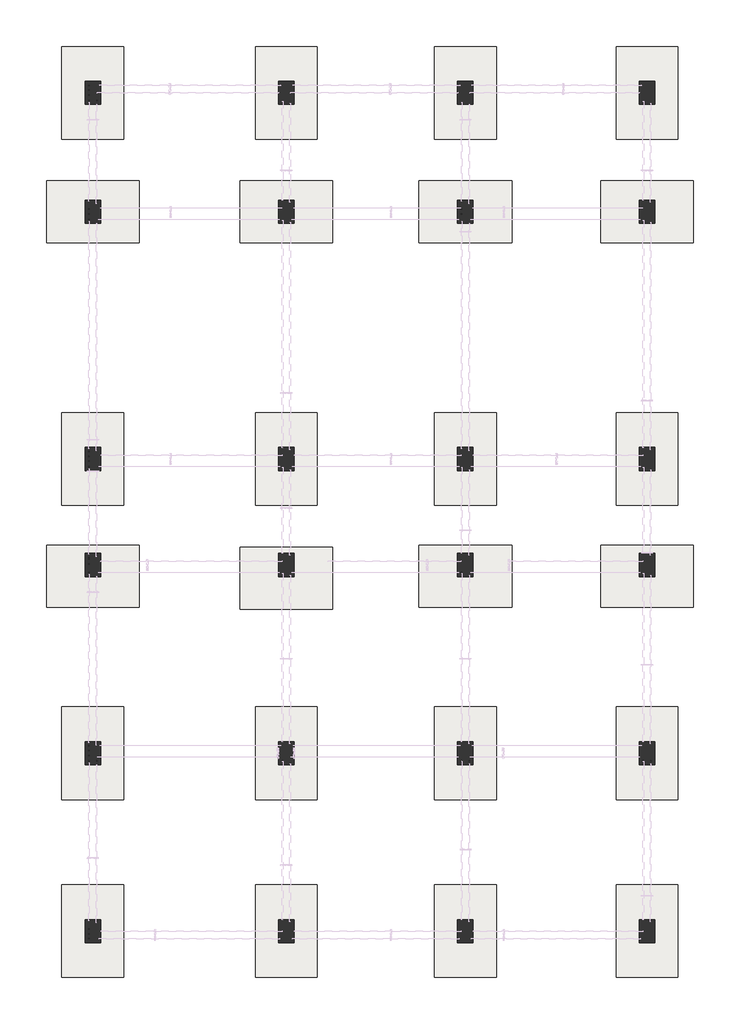
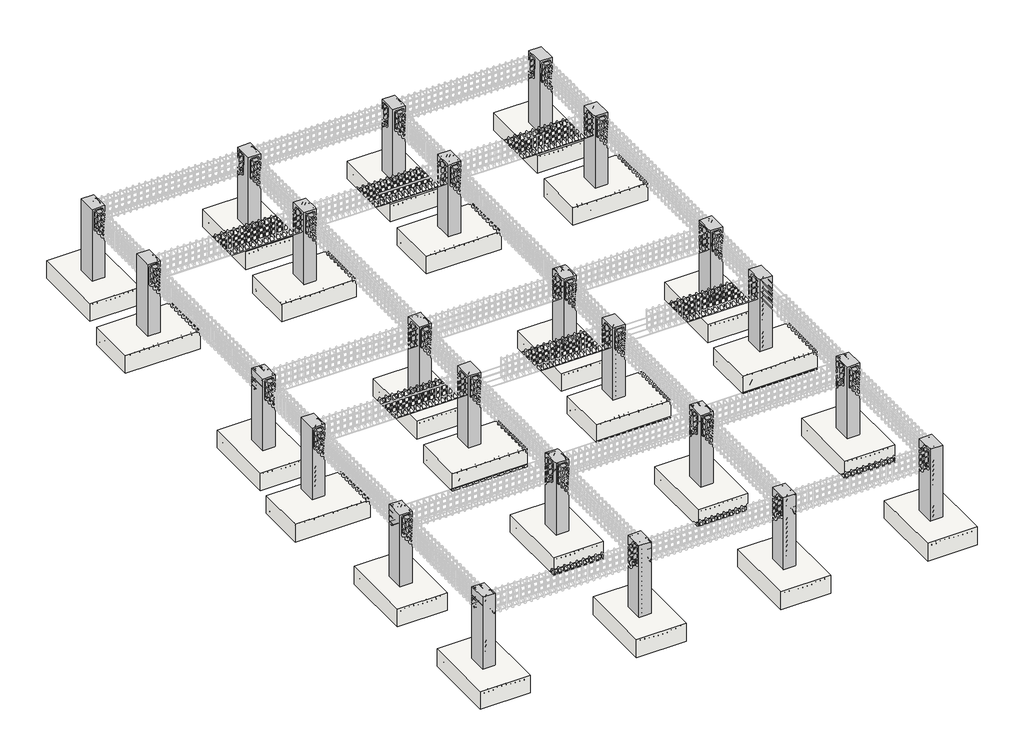
# One storey, part 1 of 20: 24 columns, 24 slabs.
"""IFC4 building model written with IfcOpenShell, lengths in millimetres."""

from ifc_helpers import new_model, si_unit, frame, origin, place, context, project, spatial, polyline, outline, extrude, faceted_brep, transform, mapped, element, save
from components import m_footing_rectangular_1800_x_1200_x_450mm_16ba7ea5

model = new_model("IFC4")

# Units and contexts
model_context = context("Model", 3, world=origin())
ifc_project = project(units=[si_unit("LENGTHUNIT", "METRE", prefix="MILLI")], contexts=[model_context])

# Site, building, storey
site = spatial("IfcSite", under=ifc_project)
building = spatial("IfcBuilding", under=site)
storey = spatial("IfcBuildingStorey", under=building, Elevation=-1828.8)

# Columns
placement = place(None, origin())
element("IfcColumn", 1, ObjectType="M_Concrete-Rectangular-Column : 300 x 450mm", at=placement, inside=storey, context=model_context, shape_type="Brep", body=[
    faceted_brep([(-5713.9412236, 10327.3331363, -1828.8), (-5713.9412236, 9877.3331363, -1828.8), (-6013.9412236, 9877.3331363, -1828.8), (-6013.9412236, 10327.3331363, -1828.8), (-5713.9412236, 10327.3331363, 0.0), (-5713.9412236, 10027.3331363, 0.0), (-5713.9412236, 9877.3331363, 0.0), (-6013.9412236, 9877.3331363, 0.0), (-6013.9412236, 10327.3331363, 0.0)], [[[0, 1, 2, 3]], [[4, 5, 6, 1, 0]], [[6, 7, 2, 1]], [[7, 8, 3, 2]], [[8, 4, 0, 3]], [[4, 8, 7, 6, 5]]]),
])
element("IfcColumn", 2, ObjectType="M_Concrete-Rectangular-Column : 300 x 450mm", at=placement, inside=storey, context=model_context, shape_type="Brep", body=[
    faceted_brep([(-5713.9412236, 8015.9331363, -1828.8), (-5713.9412236, 7565.9331363, -1828.8), (-6013.9412236, 7565.9331363, -1828.8), (-6013.9412236, 8015.9331363, -1828.8), (-5713.9412236, 8015.9331363, 0.0), (-5713.9412236, 7940.9331363, 0.0), (-5713.9412236, 7640.9331363, 0.0), (-5713.9412236, 7565.9331363, 0.0), (-6013.9412236, 7565.9331363, 0.0), (-6013.9412236, 8015.9331363, 0.0)], [[[0, 1, 2, 3]], [[4, 5, 6, 7, 1, 0]], [[7, 8, 2, 1]], [[8, 9, 3, 2]], [[9, 4, 0, 3]], [[4, 9, 8, 7, 6, 5]]]),
])
element("IfcColumn", 3, ObjectType="M_Concrete-Rectangular-Column : 300 x 450mm", at=placement, inside=storey, context=model_context, shape_type="Brep", body=[
    faceted_brep([(-5713.9412236, 3215.3331363, -1828.8), (-5713.9412236, 2765.3331363, -1828.8), (-6013.9412236, 2765.3331363, -1828.8), (-6013.9412236, 3215.3331363, -1828.8), (-5713.9412236, 3215.3331363, 0.0), (-5713.9412236, 3140.3331363, 0.0), (-5713.9412236, 2840.3331363, 0.0), (-5713.9412236, 2765.3331363, 0.0), (-6013.9412236, 2765.3331363, 0.0), (-6013.9412236, 3215.3331363, 0.0)], [[[0, 1, 2, 3]], [[4, 5, 6, 7, 1, 0]], [[7, 8, 2, 1]], [[8, 9, 3, 2]], [[9, 4, 0, 3]], [[4, 9, 8, 7, 6, 5]]]),
])
element("IfcColumn", 4, ObjectType="M_Concrete-Rectangular-Column : 300 x 450mm", at=placement, inside=storey, context=model_context, shape_type="Brep", body=[
    faceted_brep([(-6013.9412236, 707.9331363, -1828.8), (-6013.9412236, 1157.9331363, -1828.8), (-5713.9412236, 1157.9331363, -1828.8), (-5713.9412236, 707.9331363, -1828.8), (-6013.9412236, 707.9331363, 0.0), (-6013.9412236, 1157.9331363, 0.0), (-5713.9412236, 1157.9331363, 0.0), (-5713.9412236, 782.9331363, 0.0), (-5713.9412236, 707.9331363, 0.0)], [[[0, 1, 2, 3]], [[4, 5, 1, 0]], [[5, 6, 2, 1]], [[6, 7, 8, 3, 2]], [[8, 4, 0, 3]], [[4, 8, 7, 6, 5]]]),
])
element("IfcColumn", 5, ObjectType="M_Concrete-Rectangular-Column : 300 x 450mm", at=placement, inside=storey, context=model_context, shape_type="Brep", body=[
    faceted_brep([(-5713.9412236, -2499.6668637, -1828.8), (-5713.9412236, -2949.6668637, -1828.8), (-6013.9412236, -2949.6668637, -1828.8), (-6013.9412236, -2499.6668637, -1828.8), (-5713.9412236, -2499.6668637, 0.0), (-5713.9412236, -2574.6668637, 0.0), (-5713.9412236, -2874.6668637, 0.0), (-5713.9412236, -2949.6668637, 0.0), (-6013.9412236, -2949.6668637, 0.0), (-6013.9412236, -2499.6668637, 0.0)], [[[0, 1, 2, 3]], [[4, 5, 6, 7, 1, 0]], [[7, 8, 2, 1]], [[8, 9, 3, 2]], [[9, 4, 0, 3]], [[4, 9, 8, 7, 6, 5]]]),
])
element("IfcColumn", 6, ObjectType="M_Concrete-Rectangular-Column : 300 x 450mm", at=placement, inside=storey, context=model_context, shape_type="Brep", body=[
    faceted_brep([(-6013.9412236, -6404.0668637, -1828.8), (-6013.9412236, -5954.0668637, -1828.8), (-5713.9412236, -5954.0668637, -1828.8), (-5713.9412236, -6404.0668637, -1828.8), (-6013.9412236, -6404.0668637, 0.0), (-6013.9412236, -5954.0668637, 0.0), (-5713.9412236, -5954.0668637, 0.0), (-5713.9412236, -6104.0668637, 0.0), (-5713.9412236, -6404.0668637, 0.0)], [[[0, 1, 2, 3]], [[4, 5, 1, 0]], [[5, 6, 2, 1]], [[6, 7, 8, 3, 2]], [[8, 4, 0, 3]], [[4, 8, 7, 6, 5]]]),
])
element("IfcColumn", 7, ObjectType="M_Concrete-Rectangular-Column : 300 x 450mm", at=placement, inside=storey, context=model_context, shape_type="Brep", body=[
    faceted_brep([(-1952.7860107, 10327.3331363, -1828.8), (-1952.7860107, 9877.3331363, -1828.8), (-2252.7860107, 9877.3331363, -1828.8), (-2252.7860107, 10327.3331363, -1828.8), (-1952.7860107, 10327.3331363, 0.0), (-1952.7860107, 10027.3331363, 0.0), (-1952.7860107, 9877.3331363, 0.0), (-1952.7860107, 9877.3331363, -300.0), (-2252.7860107, 9877.3331363, 0.0), (-2252.7860107, 9877.3331363, -300.0), (-2252.7860107, 10027.3331363, 0.0), (-2252.7860107, 10327.3331363, 0.0)], [[[0, 1, 2, 3]], [[1, 0, 4, 5, 6, 7]], [[2, 1, 7, 6, 8, 9]], [[3, 2, 9, 8, 10, 11]], [[0, 3, 11, 4]], [[8, 6, 5, 4, 11, 10]]]),
])
element("IfcColumn", 8, ObjectType="M_Concrete-Rectangular-Column : 300 x 450mm", at=placement, inside=storey, context=model_context, shape_type="Brep", body=[
    faceted_brep([(-1952.7860107, 8015.9331363, -1828.8), (-1952.7860107, 7565.9331363, -1828.8), (-2252.7860107, 7565.9331363, -1828.8), (-2252.7860107, 8015.9331363, -1828.8), (-1952.7860107, 8015.9331363, -300.0), (-1952.7860107, 8015.9331363, 0.0), (-1952.7860107, 7940.9331363, 0.0), (-1952.7860107, 7640.9331363, 0.0), (-1952.7860107, 7565.9331363, 0.0), (-1952.7860107, 7565.9331363, -300.0), (-2252.7860107, 7565.9331363, 0.0), (-2252.7860107, 7565.9331363, -300.0), (-2252.7860107, 7640.9331363, 0.0), (-2252.7860107, 7940.9331363, 0.0), (-2252.7860107, 8015.9331363, 0.0), (-2252.7860107, 8015.9331363, -300.0)], [[[0, 1, 2, 3]], [[1, 0, 4, 5, 6, 7, 8, 9]], [[2, 1, 9, 8, 10, 11]], [[3, 2, 11, 10, 12, 13, 14, 15]], [[0, 3, 15, 14, 5, 4]], [[10, 8, 7, 6, 5, 14, 13, 12]]]),
])
element("IfcColumn", 9, ObjectType="M_Concrete-Rectangular-Column : 300 x 450mm", at=placement, inside=storey, context=model_context, shape_type="Brep", body=[
    faceted_brep([(-1952.7860107, 3215.3331363, -1828.8), (-1952.7860107, 2765.3331363, -1828.8), (-2252.7860107, 2765.3331363, -1828.8), (-2252.7860107, 3215.3331363, -1828.8), (-1952.7860107, 3215.3331363, -300.0), (-1952.7860107, 3215.3331363, 0.0), (-1952.7860107, 3140.3331363, 0.0), (-1952.7860107, 2765.3331363, 0.0), (-2252.7860107, 2765.3331363, 0.0), (-2252.7860107, 2765.3331363, -300.0), (-2252.7860107, 2840.3331363, 0.0), (-2252.7860107, 3140.3331363, 0.0), (-2252.7860107, 3215.3331363, 0.0), (-2252.7860107, 3215.3331363, -300.0)], [[[0, 1, 2, 3]], [[1, 0, 4, 5, 6, 7]], [[2, 1, 7, 8, 9]], [[3, 2, 9, 8, 10, 11, 12, 13]], [[0, 3, 13, 12, 5, 4]], [[8, 7, 6, 5, 12, 11, 10]]]),
])
element("IfcColumn", 10, ObjectType="M_Concrete-Rectangular-Column : 300 x 450mm", at=placement, inside=storey, context=model_context, shape_type="Brep", body=[
    faceted_brep([(-2252.7860107, 707.9331363, -1828.8), (-2252.7860107, 1157.9331363, -1828.8), (-1952.7860107, 1157.9331363, -1828.8), (-1952.7860107, 707.9331363, -1828.8), (-2252.7860107, 707.9331363, -300.0), (-2252.7860107, 707.9331363, 0.0), (-2252.7860107, 782.9331363, 0.0), (-2252.7860107, 1082.9331363, 0.0), (-2252.7860107, 1157.9331363, 0.0), (-2252.7860107, 1157.9331363, -300.0), (-1952.7860107, 1157.9331363, 0.0), (-1952.7860107, 782.9331363, 0.0), (-1952.7860107, 707.9331363, 0.0), (-1952.7860107, 707.9331363, -300.0)], [[[0, 1, 2, 3]], [[1, 0, 4, 5, 6, 7, 8, 9]], [[2, 1, 9, 8, 10]], [[3, 2, 10, 11, 12, 13]], [[0, 3, 13, 12, 5, 4]], [[10, 8, 7, 6, 5, 12, 11]]]),
])
element("IfcColumn", 11, ObjectType="M_Concrete-Rectangular-Column : 300 x 450mm", at=placement, inside=storey, context=model_context, shape_type="Brep", body=[
    faceted_brep([(-1952.7860107, -2499.6668637, -1828.8), (-1952.7860107, -2949.6668637, -1828.8), (-2252.7860107, -2949.6668637, -1828.8), (-2252.7860107, -2499.6668637, -1828.8), (-1952.7860107, -2499.6668637, -300.0), (-1952.7860107, -2499.6668637, 0.0), (-1952.7860107, -2574.6668637, 0.0), (-1952.7860107, -2874.6668637, 0.0), (-1952.7860107, -2949.6668637, 0.0), (-1952.7860107, -2949.6668637, -300.0), (-2252.7860107, -2949.6668637, 0.0), (-2252.7860107, -2949.6668637, -300.0), (-2252.7860107, -2874.6668637, 0.0), (-2252.7860107, -2574.6668637, 0.0), (-2252.7860107, -2499.6668637, 0.0), (-2252.7860107, -2499.6668637, -300.0)], [[[0, 1, 2, 3]], [[1, 0, 4, 5, 6, 7, 8, 9]], [[2, 1, 9, 8, 10, 11]], [[3, 2, 11, 10, 12, 13, 14, 15]], [[0, 3, 15, 14, 5, 4]], [[10, 8, 7, 6, 5, 14, 13, 12]]]),
])
element("IfcColumn", 12, ObjectType="M_Concrete-Rectangular-Column : 300 x 450mm", at=placement, inside=storey, context=model_context, shape_type="Brep", body=[
    faceted_brep([(-2252.7860107, -6404.0668637, -1828.8), (-2252.7860107, -5954.0668637, -1828.8), (-1952.7860107, -5954.0668637, -1828.8), (-1952.7860107, -6404.0668637, -1828.8), (-2252.7860107, -6404.0668637, 0.0), (-2252.7860107, -6104.0668637, 0.0), (-2252.7860107, -5954.0668637, 0.0), (-2252.7860107, -5954.0668637, -300.0), (-1952.7860107, -5954.0668637, 0.0), (-1952.7860107, -5954.0668637, -300.0), (-1952.7860107, -6104.0668637, 0.0), (-1952.7860107, -6404.0668637, 0.0)], [[[0, 1, 2, 3]], [[1, 0, 4, 5, 6, 7]], [[2, 1, 7, 6, 8, 9]], [[3, 2, 9, 8, 10, 11]], [[0, 3, 11, 4]], [[8, 6, 5, 4, 11, 10]]]),
])
element("IfcColumn", 13, ObjectType="M_Concrete-Rectangular-Column : 300 x 450mm", at=placement, inside=storey, context=model_context, shape_type="Brep", body=[
    faceted_brep([(1527.0139893, 10327.3331363, -1828.8), (1527.0139893, 9877.3331363, -1828.8), (1227.0139893, 9877.3331363, -1828.8), (1227.0139893, 10327.3331363, -1828.8), (1527.0139893, 10327.3331363, 0.0), (1527.0139893, 10027.3331363, 0.0), (1527.0139893, 9877.3331363, 0.0), (1527.0139893, 9877.3331363, -300.0), (1227.0139893, 9877.3331363, 0.0), (1227.0139893, 9877.3331363, -300.0), (1227.0139893, 10027.3331363, 0.0), (1227.0139893, 10327.3331363, 0.0)], [[[0, 1, 2, 3]], [[1, 0, 4, 5, 6, 7]], [[2, 1, 7, 6, 8, 9]], [[3, 2, 9, 8, 10, 11]], [[0, 3, 11, 4]], [[8, 6, 5, 4, 11, 10]]]),
])
element("IfcColumn", 14, ObjectType="M_Concrete-Rectangular-Column : 300 x 450mm", at=placement, inside=storey, context=model_context, shape_type="Brep", body=[
    faceted_brep([(1527.0139893, 8015.9331363, -1828.8), (1527.0139893, 7565.9331363, -1828.8), (1227.0139893, 7565.9331363, -1828.8), (1227.0139893, 8015.9331363, -1828.8), (1527.0139893, 8015.9331363, -300.0), (1527.0139893, 8015.9331363, 0.0), (1527.0139893, 7940.9331363, 0.0), (1527.0139893, 7640.9331363, 0.0), (1527.0139893, 7565.9331363, 0.0), (1527.0139893, 7565.9331363, -300.0), (1227.0139893, 7565.9331363, 0.0), (1227.0139893, 7565.9331363, -300.0), (1227.0139893, 7640.9331363, 0.0), (1227.0139893, 7940.9331363, 0.0), (1227.0139893, 8015.9331363, 0.0), (1227.0139893, 8015.9331363, -300.0)], [[[0, 1, 2, 3]], [[1, 0, 4, 5, 6, 7, 8, 9]], [[2, 1, 9, 8, 10, 11]], [[3, 2, 11, 10, 12, 13, 14, 15]], [[0, 3, 15, 14, 5, 4]], [[10, 8, 7, 6, 5, 14, 13, 12]]]),
])
element("IfcColumn", 15, ObjectType="M_Concrete-Rectangular-Column : 300 x 450mm", at=placement, inside=storey, context=model_context, shape_type="Brep", body=[
    faceted_brep([(1527.0139893, 3215.3331363, -1828.8), (1527.0139893, 2765.3331363, -1828.8), (1227.0139893, 2765.3331363, -1828.8), (1227.0139893, 3215.3331363, -1828.8), (1527.0139893, 3215.3331363, -300.0), (1527.0139893, 3215.3331363, 0.0), (1527.0139893, 3140.3331363, 0.0), (1527.0139893, 2765.3331363, 0.0), (1227.0139893, 2765.3331363, 0.0), (1227.0139893, 2765.3331363, -300.0), (1227.0139893, 2840.3331363, 0.0), (1227.0139893, 3140.3331363, 0.0), (1227.0139893, 3215.3331363, 0.0), (1227.0139893, 3215.3331363, -300.0)], [[[0, 1, 2, 3]], [[1, 0, 4, 5, 6, 7]], [[2, 1, 7, 8, 9]], [[3, 2, 9, 8, 10, 11, 12, 13]], [[0, 3, 13, 12, 5, 4]], [[8, 7, 6, 5, 12, 11, 10]]]),
])
element("IfcColumn", 16, ObjectType="M_Concrete-Rectangular-Column : 300 x 450mm", at=placement, inside=storey, context=model_context, shape_type="Brep", body=[
    faceted_brep([(1227.0139893, 707.9331363, -1828.8), (1227.0139893, 1157.9331363, -1828.8), (1527.0139893, 1157.9331363, -1828.8), (1527.0139893, 707.9331363, -1828.8), (1227.0139893, 707.9331363, -300.0), (1227.0139893, 707.9331363, 0.0), (1227.0139893, 782.9331363, 0.0), (1227.0139893, 1082.9331363, 0.0), (1227.0139893, 1157.9331363, 0.0), (1227.0139893, 1157.9331363, -300.0), (1527.0139893, 1157.9331363, 0.0), (1527.0139893, 782.9331363, 0.0), (1527.0139893, 707.9331363, 0.0), (1527.0139893, 707.9331363, -300.0)], [[[0, 1, 2, 3]], [[1, 0, 4, 5, 6, 7, 8, 9]], [[2, 1, 9, 8, 10]], [[3, 2, 10, 11, 12, 13]], [[0, 3, 13, 12, 5, 4]], [[10, 8, 7, 6, 5, 12, 11]]]),
])
element("IfcColumn", 17, ObjectType="M_Concrete-Rectangular-Column : 300 x 450mm", at=placement, inside=storey, context=model_context, shape_type="Brep", body=[
    faceted_brep([(1527.0139893, -2499.6668637, -1828.8), (1527.0139893, -2949.6668637, -1828.8), (1227.0139893, -2949.6668637, -1828.8), (1227.0139893, -2499.6668637, -1828.8), (1527.0139893, -2499.6668637, -300.0), (1527.0139893, -2499.6668637, 0.0), (1527.0139893, -2574.6668637, 0.0), (1527.0139893, -2874.6668637, 0.0), (1527.0139893, -2949.6668637, 0.0), (1527.0139893, -2949.6668637, -300.0), (1227.0139893, -2949.6668637, 0.0), (1227.0139893, -2949.6668637, -300.0), (1227.0139893, -2874.6668637, 0.0), (1227.0139893, -2574.6668637, 0.0), (1227.0139893, -2499.6668637, 0.0), (1227.0139893, -2499.6668637, -300.0)], [[[0, 1, 2, 3]], [[1, 0, 4, 5, 6, 7, 8, 9]], [[2, 1, 9, 8, 10, 11]], [[3, 2, 11, 10, 12, 13, 14, 15]], [[0, 3, 15, 14, 5, 4]], [[10, 8, 7, 6, 5, 14, 13, 12]]]),
])
element("IfcColumn", 18, ObjectType="M_Concrete-Rectangular-Column : 300 x 450mm", at=placement, inside=storey, context=model_context, shape_type="Brep", body=[
    faceted_brep([(1227.0139893, -6404.0668637, -1828.8), (1227.0139893, -5954.0668637, -1828.8), (1527.0139893, -5954.0668637, -1828.8), (1527.0139893, -6404.0668637, -1828.8), (1227.0139893, -6404.0668637, 0.0), (1227.0139893, -6104.0668637, 0.0), (1227.0139893, -5954.0668637, 0.0), (1227.0139893, -5954.0668637, -300.0), (1527.0139893, -5954.0668637, 0.0), (1527.0139893, -5954.0668637, -300.0), (1527.0139893, -6104.0668637, 0.0), (1527.0139893, -6404.0668637, 0.0)], [[[0, 1, 2, 3]], [[1, 0, 4, 5, 6, 7]], [[2, 1, 7, 6, 8, 9]], [[3, 2, 9, 8, 10, 11]], [[0, 3, 11, 4]], [[8, 6, 5, 4, 11, 10]]]),
])
element("IfcColumn", 19, ObjectType="M_Concrete-Rectangular-Column : 300 x 450mm", at=placement, inside=storey, context=model_context, shape_type="Brep", body=[
    faceted_brep([(5057.6139893, 10327.3331363, -1828.8), (5057.6139893, 9877.3331363, -1828.8), (4757.6139893, 9877.3331363, -1828.8), (4757.6139893, 10327.3331363, -1828.8), (5057.6139893, 10327.3331363, 0.0), (5057.6139893, 9877.3331363, 0.0), (4757.6139893, 9877.3331363, 0.0), (4757.6139893, 10027.3331363, 0.0), (4757.6139893, 10327.3331363, 0.0)], [[[0, 1, 2, 3]], [[4, 5, 1, 0]], [[5, 6, 2, 1]], [[6, 7, 8, 3, 2]], [[8, 4, 0, 3]], [[4, 8, 7, 6, 5]]]),
])
element("IfcColumn", 20, ObjectType="M_Concrete-Rectangular-Column : 300 x 450mm", at=placement, inside=storey, context=model_context, shape_type="Brep", body=[
    faceted_brep([(5057.6139893, 8015.9331363, -1828.8), (5057.6139893, 7565.9331363, -1828.8), (4757.6139893, 7565.9331363, -1828.8), (4757.6139893, 8015.9331363, -1828.8), (5057.6139893, 8015.9331363, 0.0), (5057.6139893, 7565.9331363, 0.0), (4757.6139893, 7565.9331363, 0.0), (4757.6139893, 7640.9331363, 0.0), (4757.6139893, 7940.9331363, 0.0), (4757.6139893, 8015.9331363, 0.0)], [[[0, 1, 2, 3]], [[4, 5, 1, 0]], [[5, 6, 2, 1]], [[6, 7, 8, 9, 3, 2]], [[9, 4, 0, 3]], [[4, 9, 8, 7, 6, 5]]]),
])
element("IfcColumn", 21, ObjectType="M_Concrete-Rectangular-Column : 300 x 450mm", at=placement, inside=storey, context=model_context, shape_type="Brep", body=[
    faceted_brep([(5057.6139893, 3215.3331363, -1828.8), (5057.6139893, 2765.3331363, -1828.8), (4757.6139893, 2765.3331363, -1828.8), (4757.6139893, 3215.3331363, -1828.8), (5057.6139893, 3215.3331363, 0.0), (5057.6139893, 2765.3331363, 0.0), (4757.6139893, 2765.3331363, 0.0), (4757.6139893, 2840.3331363, 0.0), (4757.6139893, 3140.3331363, 0.0), (4757.6139893, 3215.3331363, 0.0)], [[[0, 1, 2, 3]], [[4, 5, 1, 0]], [[5, 6, 2, 1]], [[6, 7, 8, 9, 3, 2]], [[9, 4, 0, 3]], [[4, 9, 8, 7, 6, 5]]]),
])
element("IfcColumn", 22, ObjectType="M_Concrete-Rectangular-Column : 300 x 450mm", at=placement, inside=storey, context=model_context, shape_type="Brep", body=[
    faceted_brep([(4757.6139893, 707.9331363, -1828.8), (4757.6139893, 1157.9331363, -1828.8), (5057.6139893, 1157.9331363, -1828.8), (5057.6139893, 707.9331363, -1828.8), (4757.6139893, 707.9331363, 0.0), (4757.6139893, 782.9331363, 0.0), (4757.6139893, 1082.9331363, 0.0), (4757.6139893, 1157.9331363, 0.0), (5057.6139893, 1157.9331363, 0.0), (5057.6139893, 707.9331363, 0.0)], [[[0, 1, 2, 3]], [[4, 5, 6, 7, 1, 0]], [[7, 8, 2, 1]], [[8, 9, 3, 2]], [[9, 4, 0, 3]], [[4, 9, 8, 7, 6, 5]]]),
])
element("IfcColumn", 23, ObjectType="M_Concrete-Rectangular-Column : 300 x 450mm", at=placement, inside=storey, context=model_context, shape_type="Brep", body=[
    faceted_brep([(5057.6139893, -2499.6668637, -1828.8), (5057.6139893, -2949.6668637, -1828.8), (4757.6139893, -2949.6668637, -1828.8), (4757.6139893, -2499.6668637, -1828.8), (5057.6139893, -2499.6668637, 0.0), (5057.6139893, -2949.6668637, 0.0), (4757.6139893, -2949.6668637, 0.0), (4757.6139893, -2874.6668637, 0.0), (4757.6139893, -2574.6668637, 0.0), (4757.6139893, -2499.6668637, 0.0)], [[[0, 1, 2, 3]], [[4, 5, 1, 0]], [[5, 6, 2, 1]], [[6, 7, 8, 9, 3, 2]], [[9, 4, 0, 3]], [[4, 9, 8, 7, 6, 5]]]),
])
element("IfcColumn", 24, ObjectType="M_Concrete-Rectangular-Column : 300 x 450mm", at=placement, inside=storey, context=model_context, shape_type="Brep", body=[
    faceted_brep([(4757.6139893, -6404.0668637, -1828.8), (4757.6139893, -5954.0668637, -1828.8), (5057.6139893, -5954.0668637, -1828.8), (5057.6139893, -6404.0668637, -1828.8), (4757.6139893, -6404.0668637, 0.0), (4757.6139893, -6104.0668637, 0.0), (4757.6139893, -5954.0668637, 0.0), (5057.6139893, -5954.0668637, 0.0), (5057.6139893, -6404.0668637, 0.0)], [[[0, 1, 2, 3]], [[4, 5, 6, 1, 0]], [[6, 7, 2, 1]], [[7, 8, 3, 2]], [[8, 4, 0, 3]], [[4, 8, 7, 6, 5]]]),
])

# Slabs
element("IfcSlab", 25, ObjectType="M_Footing-Rectangular : 1800 x 1200 x 450mm", at=placement, inside=storey, context=model_context, shape_type="SweptSolid", body=[
    extrude(outline(polyline([(-5263.9412236, 11002.3331363), (-5263.9412236, 9202.3331363), (-6463.9412236, 9202.3331363), (-6463.9412236, 11002.3331363), (-5263.9412236, 11002.3331363)])), frame((0.0, 0.0, -2278.8), z_axis=(0.0, 0.0, 1.0), x_axis=(1.0, 0.0, 0.0)), (0.0, 0.0, 1.0), 450.0),
])
element("IfcSlab", 26, ObjectType="M_Footing-Rectangular : 1800 x 1200 x 450mm", at=placement, inside=storey, context=model_context, shape_type="SweptSolid", body=[
    extrude(outline(polyline([(-5263.9412236, 3890.3331363), (-5263.9412236, 2090.3331363), (-6463.9412236, 2090.3331363), (-6463.9412236, 3890.3331363), (-5263.9412236, 3890.3331363)])), frame((0.0, 0.0, -2278.8), z_axis=(0.0, 0.0, 1.0), x_axis=(1.0, 0.0, 0.0)), (0.0, 0.0, 1.0), 450.0),
])
element("IfcSlab", 27, ObjectType="M_Footing-Rectangular : 1800 x 1200 x 450mm", at=placement, inside=storey, context=model_context, shape_type="SweptSolid", body=[
    extrude(outline(polyline([(-5263.9412236, -1824.6668637), (-5263.9412236, -3624.6668637), (-6463.9412236, -3624.6668637), (-6463.9412236, -1824.6668637), (-5263.9412236, -1824.6668637)])), frame((0.0, 0.0, -2278.8), z_axis=(0.0, 0.0, 1.0), x_axis=(1.0, 0.0, 0.0)), (0.0, 0.0, 1.0), 450.0),
])
element("IfcSlab", 28, ObjectType="M_Footing-Rectangular : 1800 x 1200 x 450mm", at=placement, inside=storey, context=model_context, shape_type="SweptSolid", body=[
    extrude(outline(polyline([(-6463.9412236, -7079.0668637), (-6463.9412236, -5279.0668637), (-5263.9412236, -5279.0668637), (-5263.9412236, -7079.0668637), (-6463.9412236, -7079.0668637)])), frame((0.0, 0.0, -2278.8), z_axis=(0.0, 0.0, 1.0), x_axis=(1.0, 0.0, 0.0)), (0.0, 0.0, 1.0), 450.0),
])
element("IfcSlab", 29, ObjectType="M_Footing-Rectangular : 1800 x 1200 x 450mm", at=placement, inside=storey, context=model_context, shape_type="SweptSolid", body=[
    extrude(outline(polyline([(-1502.7860107, 11002.3331363), (-1502.7860107, 9202.3331363), (-2702.7860107, 9202.3331363), (-2702.7860107, 11002.3331363), (-1502.7860107, 11002.3331363)])), frame((0.0, 0.0, -2278.8), z_axis=(0.0, 0.0, 1.0), x_axis=(1.0, 0.0, 0.0)), (0.0, 0.0, 1.0), 450.0),
])
element("IfcSlab", 30, ObjectType="M_Footing-Rectangular : 1800 x 1200 x 450mm", at=placement, inside=storey, context=model_context, shape_type="SweptSolid", body=[
    extrude(outline(polyline([(-2702.7860107, -7079.0668637), (-2702.7860107, -5279.0668637), (-1502.7860107, -5279.0668637), (-1502.7860107, -7079.0668637), (-2702.7860107, -7079.0668637)])), frame((0.0, 0.0, -2278.8), z_axis=(0.0, 0.0, 1.0), x_axis=(1.0, 0.0, 0.0)), (0.0, 0.0, 1.0), 450.0),
])
element("IfcSlab", 31, ObjectType="M_Footing-Rectangular : 1800 x 1200 x 450mm", at=placement, inside=storey, context=model_context, shape_type="SweptSolid", body=[
    extrude(outline(polyline([(1977.0139893, 11002.3331363), (1977.0139893, 9202.3331363), (777.0139893, 9202.3331363), (777.0139893, 11002.3331363), (1977.0139893, 11002.3331363)])), frame((0.0, 0.0, -2278.8), z_axis=(0.0, 0.0, 1.0), x_axis=(1.0, 0.0, 0.0)), (0.0, 0.0, 1.0), 450.0),
])
element("IfcSlab", 32, ObjectType="M_Footing-Rectangular : 1800 x 1200 x 450mm", at=placement, inside=storey, context=model_context, shape_type="SweptSolid", body=[
    extrude(outline(polyline([(777.0139893, -7079.0668637), (777.0139893, -5279.0668637), (1977.0139893, -5279.0668637), (1977.0139893, -7079.0668637), (777.0139893, -7079.0668637)])), frame((0.0, 0.0, -2278.8), z_axis=(0.0, 0.0, 1.0), x_axis=(1.0, 0.0, 0.0)), (0.0, 0.0, 1.0), 450.0),
])
element("IfcSlab", 33, ObjectType="M_Footing-Rectangular : 1800 x 1200 x 450mm", at=placement, inside=storey, context=model_context, shape_type="SweptSolid", body=[
    extrude(outline(polyline([(5507.6139893, 11002.3331363), (5507.6139893, 9202.3331363), (4307.6139893, 9202.3331363), (4307.6139893, 11002.3331363), (5507.6139893, 11002.3331363)])), frame((0.0, 0.0, -2278.8), z_axis=(0.0, 0.0, 1.0), x_axis=(1.0, 0.0, 0.0)), (0.0, 0.0, 1.0), 450.0),
])
element("IfcSlab", 34, ObjectType="M_Footing-Rectangular : 1800 x 1200 x 450mm", at=placement, inside=storey, context=model_context, shape_type="SweptSolid", body=[
    extrude(outline(polyline([(5507.6139893, 3890.3331363), (5507.6139893, 2090.3331363), (4307.6139893, 2090.3331363), (4307.6139893, 3890.3331363), (5507.6139893, 3890.3331363)])), frame((0.0, 0.0, -2278.8), z_axis=(0.0, 0.0, 1.0), x_axis=(1.0, 0.0, 0.0)), (0.0, 0.0, 1.0), 450.0),
])
element("IfcSlab", 35, ObjectType="M_Footing-Rectangular : 1800 x 1200 x 450mm", at=placement, inside=storey, context=model_context, shape_type="SweptSolid", body=[
    extrude(outline(polyline([(5507.6139893, -1824.6668637), (5507.6139893, -3624.6668637), (4307.6139893, -3624.6668637), (4307.6139893, -1824.6668637), (5507.6139893, -1824.6668637)])), frame((0.0, 0.0, -2278.8), z_axis=(0.0, 0.0, 1.0), x_axis=(1.0, 0.0, 0.0)), (0.0, 0.0, 1.0), 450.0),
])
element("IfcSlab", 36, ObjectType="M_Footing-Rectangular : 1800 x 1200 x 450mm", at=placement, inside=storey, context=model_context, shape_type="SweptSolid", body=[
    extrude(outline(polyline([(4307.6139893, -7079.0668637), (4307.6139893, -5279.0668637), (5507.6139893, -5279.0668637), (5507.6139893, -7079.0668637), (4307.6139893, -7079.0668637)])), frame((0.0, 0.0, -2278.8), z_axis=(0.0, 0.0, 1.0), x_axis=(1.0, 0.0, 0.0)), (0.0, 0.0, 1.0), 450.0),
])
element("IfcSlab", 37, ObjectType="M_Footing-Rectangular : 1800 x 1200 x 450mm", at=placement, inside=storey, context=model_context, shape_type="SweptSolid", body=[
    extrude(outline(polyline([(-6763.9412236, 1312.9331363), (-4963.9412236, 1312.9331363), (-4963.9412236, 112.9331363), (-6763.9412236, 112.9331363), (-6763.9412236, 1312.9331363)])), frame((0.0, 0.0, -2278.8), z_axis=(0.0, 0.0, 1.0), x_axis=(1.0, 0.0, 0.0)), (0.0, 0.0, 1.0), 450.0),
])
element("IfcSlab", 38, ObjectType="M_Footing-Rectangular : 1800 x 1200 x 450mm", at=placement, inside=storey, context=model_context, shape_type="SweptSolid", body=[
    extrude(outline(polyline([(-3002.7860107, 1272.9331363), (-1202.7860107, 1272.9331363), (-1202.7860107, 72.9331363), (-3002.7860107, 72.9331363), (-3002.7860107, 1272.9331363)])), frame((0.0, 0.0, -2278.8), z_axis=(0.0, 0.0, 1.0), x_axis=(1.0, 0.0, 0.0)), (0.0, 0.0, 1.0), 450.0),
])
element("IfcSlab", 39, ObjectType="M_Footing-Rectangular : 1800 x 1200 x 450mm", at=placement, inside=storey, context=model_context, shape_type="SweptSolid", body=[
    extrude(outline(polyline([(477.0139893, 1312.9331363), (2277.0139893, 1312.9331363), (2277.0139893, 112.9331363), (477.0139893, 112.9331363), (477.0139893, 1312.9331363)])), frame((0.0, 0.0, -2278.8), z_axis=(0.0, 0.0, 1.0), x_axis=(1.0, 0.0, 0.0)), (0.0, 0.0, 1.0), 450.0),
])
element("IfcSlab", 40, ObjectType="M_Footing-Rectangular : 1800 x 1200 x 450mm", at=placement, inside=storey, context=model_context, shape_type="SweptSolid", body=[
    extrude(outline(polyline([(4007.6139893, 1312.9331363), (5807.6139893, 1312.9331363), (5807.6139893, 112.9331363), (4007.6139893, 112.9331363), (4007.6139893, 1312.9331363)])), frame((0.0, 0.0, -2278.8), z_axis=(0.0, 0.0, 1.0), x_axis=(1.0, 0.0, 0.0)), (0.0, 0.0, 1.0), 450.0),
])
element("IfcSlab", 41, ObjectType="M_Footing-Rectangular : 1800 x 1200 x 450mm", at=placement, inside=storey, context=model_context, shape_type="SweptSolid", body=[
    extrude(outline(polyline([(4007.6139893, 8390.9331363), (5807.6139893, 8390.9331363), (5807.6139893, 7190.9331363), (4007.6139893, 7190.9331363), (4007.6139893, 8390.9331363)])), frame((0.0, 0.0, -2278.8), z_axis=(0.0, 0.0, 1.0), x_axis=(1.0, 0.0, 0.0)), (0.0, 0.0, 1.0), 450.0),
])
element("IfcSlab", 42, ObjectType="M_Footing-Rectangular : 1800 x 1200 x 450mm", at=placement, inside=storey, context=model_context, shape_type="SweptSolid", body=[
    extrude(outline(polyline([(477.0139893, 8390.9331363), (2277.0139893, 8390.9331363), (2277.0139893, 7190.9331363), (477.0139893, 7190.9331363), (477.0139893, 8390.9331363)])), frame((0.0, 0.0, -2278.8), z_axis=(0.0, 0.0, 1.0), x_axis=(1.0, 0.0, 0.0)), (0.0, 0.0, 1.0), 450.0),
])
element("IfcSlab", 43, ObjectType="M_Footing-Rectangular : 1800 x 1200 x 450mm", at=placement, inside=storey, context=model_context, shape_type="SweptSolid", body=[
    extrude(outline(polyline([(-3002.7860107, 8390.9331363), (-1202.7860107, 8390.9331363), (-1202.7860107, 7190.9331363), (-3002.7860107, 7190.9331363), (-3002.7860107, 8390.9331363)])), frame((0.0, 0.0, -2278.8), z_axis=(0.0, 0.0, 1.0), x_axis=(1.0, 0.0, 0.0)), (0.0, 0.0, 1.0), 450.0),
])
element("IfcSlab", 44, ObjectType="M_Footing-Rectangular : 1800 x 1200 x 450mm", at=placement, inside=storey, context=model_context, shape_type="SweptSolid", body=[
    extrude(outline(polyline([(-6763.9412236, 8390.9331363), (-4963.9412236, 8390.9331363), (-4963.9412236, 7190.9331363), (-6763.9412236, 7190.9331363), (-6763.9412236, 8390.9331363)])), frame((0.0, 0.0, -2278.8), z_axis=(0.0, 0.0, 1.0), x_axis=(1.0, 0.0, 0.0)), (0.0, 0.0, 1.0), 450.0),
])
m_footing_rectangular_1800_x_1200_x_450mm_shape = m_footing_rectangular_1800_x_1200_x_450mm_16ba7ea5(model_context)
element("IfcSlab", 45, ObjectType="M_Footing-Rectangular : 1800 x 1200 x 450mm", at=placement, inside=storey, context=model_context, shape_type="MappedRepresentation", body=[
    mapped(m_footing_rectangular_1800_x_1200_x_450mm_shape, transform((-2102.7860107, 2990.3331363, -1828.8), x_axis=(1.0, 0.0, 0.0), y_axis=(0.0, 1.0, 0.0), z_axis=(0.0, 0.0, 1.0))),
])
element("IfcSlab", 46, ObjectType="M_Footing-Rectangular : 1800 x 1200 x 450mm", at=placement, inside=storey, context=model_context, shape_type="MappedRepresentation", body=[
    mapped(m_footing_rectangular_1800_x_1200_x_450mm_shape, transform((-2102.7860107, -2724.6668637, -1828.8), x_axis=(1.0, 0.0, 0.0), y_axis=(0.0, 1.0, 0.0), z_axis=(0.0, 0.0, 1.0))),
])
element("IfcSlab", 47, ObjectType="M_Footing-Rectangular : 1800 x 1200 x 450mm", at=placement, inside=storey, context=model_context, shape_type="MappedRepresentation", body=[
    mapped(m_footing_rectangular_1800_x_1200_x_450mm_shape, transform((1377.0139893, 2990.3331363, -1828.8), x_axis=(1.0, 0.0, 0.0), y_axis=(0.0, 1.0, 0.0), z_axis=(0.0, 0.0, 1.0))),
])
element("IfcSlab", 48, ObjectType="M_Footing-Rectangular : 1800 x 1200 x 450mm", at=placement, inside=storey, context=model_context, shape_type="MappedRepresentation", body=[
    mapped(m_footing_rectangular_1800_x_1200_x_450mm_shape, transform((1377.0139893, -2724.6668637, -1828.8), x_axis=(1.0, 0.0, 0.0), y_axis=(0.0, 1.0, 0.0), z_axis=(0.0, 0.0, 1.0))),
])

save(model, "model.ifc")

# Revit data of these elements
# Grids (mm)
#   "1": line (-5863.941, -8762.843) -> (-5863.941, 13659.904)
#   "2": line (-2102.786, 13642.038) -> (-2102.786, -8388.552)
#   "3": line (1377.014, -8572.206) -> (1377.014, 13659.904)
#   "4": line (4907.614, -8377.096) -> (4907.614, 13659.904)
#   "A": line (7306.725, 10102.333) -> (-9174.96, 10102.333)
#   "B": line (7544.446, 7790.933) -> (-9146.428, 7790.933)
#   "C": line (7544.446, 2990.333) -> (-9521.879, 2990.333)
#   "D": line (-9174.96, 932.933) -> (7544.446, 932.933)
#   "E": line (7544.446, -2724.667) -> (-9188.801, -2724.667)
#   "F": line (-9174.96, -6179.067) -> (7544.446, -6179.067)
# Type "M_Concrete-Rectangular-Column : 300 x 450mm"
#   b = 0' - 11.81102"
#   h = 1' - 5.71654"
#   Structural Material [instance default] = Concrete, Cast-in-Place gray
# Type "M_Footing-Rectangular : 1800 x 1200 x 450mm"
#   Width = 3' - 11.24409"
#   Length = 5' - 10.86614"
#   Foundation Thickness = 1' - 5.71654"
#   Structural Material [instance default] = Concrete, Cast-in-Place gray
#   Assembly Code = ""
# Elements 1, 2, 3, 4, 5, 6, 7, 8, 9, 10, 11, 12, 13, 14, 15, 16, 17, 18, 19, 20, 21, 22, 23, 24 (IfcColumn, "M_Concrete-Rectangular-Column : 300 x 450mm")
#   Structural Material = Concrete, Cast-in-Place gray
#   Phase Created = New Construction
#   Materials on its faces: "Concrete, Cast-in-Place gray"
# Elements 25, 26, 27, 28, 29, 30, 31, 32, 33, 34, 35, 36, 37, 38, 39, 40, 41, 42, 43, 44, 45, 46, 47, 48 (IfcSlab, "M_Footing-Rectangular : 1800 x 1200 x 450mm")
#   Structural Material = Concrete, Cast-in-Place gray
#   Phase Created = New Construction
#   Materials on its faces: "Concrete, Cast-in-Place gray"
# Materials
#   "Concrete, Cast-in-Place gray": class "Concrete", colour RGB 192 192 192, transparency 0, Description = "Cast-in-place concrete", Cost = 0
